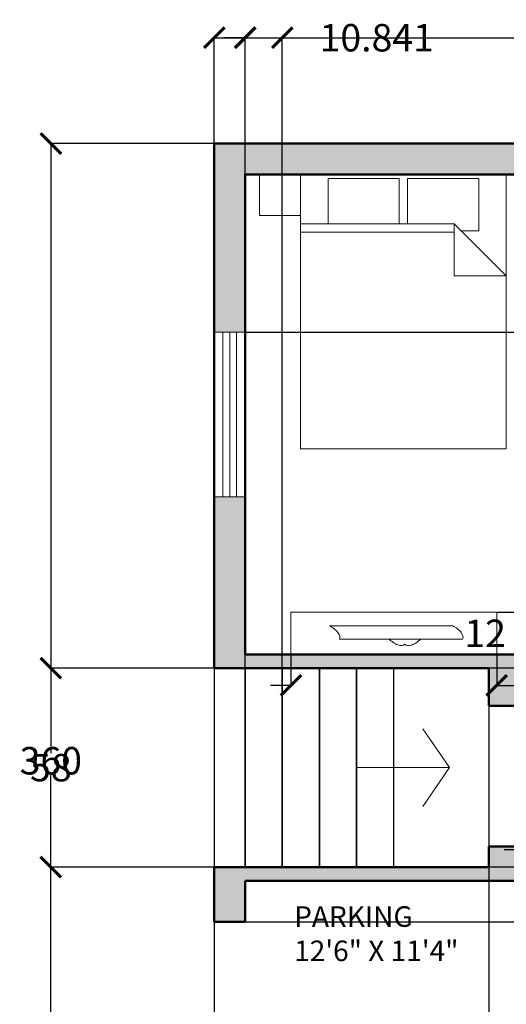
# Model space of a CAD drawing. Units: inches. Extents: x -30 to 744, y -375 to 57.
# Tile 2 of 8: x -26 to 116, y -230 to 57. Entities that reach past the tile are written whole.
import ezdxf

# ---------------------------------------------------------------- set-up
doc = ezdxf.new("R2010")
doc.units = ezdxf.units.IN
doc.header["$MEASUREMENT"] = 0
for name, color, linetype, lineweight in [('A-ANNO-DIMS', 2, 'Continuous', 18), ('A-ANNO-SYMB', 7, 'Continuous', 18), ('A-AREA-IDEN', 7, 'Continuous', 25), ('A-DOOR', 3, 'Continuous', 25), ('A-FLOR-STRS', 7, 'Continuous', 25), ('A-FURN', 8, 'Continuous', 18), ('A-GLAZ', 4, 'Continuous', 18), ('A-WALL', 7, 'Continuous', 50)]:
    doc.layers.add(name, color=color, linetype=linetype, lineweight=lineweight)
doc.layers.add('A-WALL-PATT', color=251, linetype='Continuous', lineweight=13, true_color=0x636466)
doc.styles.get("Standard").update_dxf_attribs({"font": 'arial.ttf'})
doc.dimstyles.get("Standard").update_dxf_attribs({"dimtxt": 8, "dimasz": 6, "dimexe": 0.18, "dimexo": 0.0625, "dimgap": 0.09, "dimtad": 0, "dimtih": 1, "dimtoh": 1, "dimdec": 0, "dimzin": 0, "dimdsep": 46, "dimlunit": 4, "dimtxsty": 'Standard', "dimblk": 'ARCHTICK', "dimcen": 0.09, "dimadec": 0, "dimazin": 0, "dimtfac": 1, "dimtdec": 0, "dimtofl": 0, "dimtmove": 0, "dimatfit": 1, "dimldrblk": 'ARCHTICK', "dimfxl": 1, "dimtolj": 1, "dimtzin": 0, "dimarcsym": 0})

# ---------------------------------------------------------------- blocks, each defined once
blk = doc.blocks.new('*U2')
for p, q in [((0, 0), (0, -6)), ((40, 0), (40, -6))]:
    blk.add_line(p, q)
blk.add_lwpolyline([(0, 0), (34.64, 20), (35.52, 18.48), (0.87, -1.52)], close=True)
blk.add_arc((0, 0), 40, 0, 30)
blk = doc.blocks.new('Bed - Queen')
for p, q in [((0, -80.00003), (0, 0)), ((0, 0), (59.99999, 0)), ((59.99999, 0), (59.99999, -80.00003)), ((7.99999, -1.2), (28.79998, -1.2)), ((7.99999, -14.4), (7.99999, -1.2)), ((28.79998, -1.2), (28.79998, -14.4)), ((31.19999, -1.2), (51.99999, -1.2)), ((31.19999, -14.4), (31.19999, -1.2)), ((51.99999, -1.2), (51.99999, -16.4)), ((0, -14.4), (44.8, -14.4)), ((44.8, -16.8), (0, -16.8)), ((59.99999, -29.6), (44.8, -14.4)), ((44.8, -14.4), (44.8, -29.6)), ((51.99999, -16.4), (46.79936, -16.4)), ((44.8, -29.6), (59.99999, -29.6)), ((59.99999, -80.00003), (0, -80.00003))]:
    blk.add_line(p, q)
blk = doc.blocks.new('WIN-48IN')
for p, q in [((0, 0), (0, 48)), ((0, 48), (9, 48)), ((2.5, 48), (2.5, 0)), ((4.5, 48), (4.5, 0)), ((6.5, 48), (6.5, 0)), ((9, 48), (9, 0)), ((9, 48), (9, 0)), ((9, 0), (0, 0))]:
    blk.add_line(p, q)
blk = doc.blocks.new('TV-CONSOLE-60IN')
blk.add_lwpolyline([(0, 12.35), (60, 12.35), (60, 0), (0, 0)], close=True)
for points in [[(11.23, 8.37), (47.17, 8.37)], [(50.06, 4.48), (14.12, 4.48)]]:
    blk.add_lwpolyline(points)
for centre, major_axis in [((10.57, 6.42), (3.55, -1.95)), ((46.51, 6.42), (3.55, -1.95)), ((36.16, 5.7), (-3.02, -2.7))]:
    blk.add_ellipse(centre, major_axis=major_axis, ratio=0.501579, start_param=0, end_param=1.660459)
at = {"extrusion": (0, 0, -1)}
blk.add_ellipse((30.21, 5.79), major_axis=(2.93, -2.79), ratio=0.501579, start_param=0, end_param=1.660459, dxfattribs=at)
blk = doc.blocks.new('NIGHTSTAND-12IN')
blk.add_lwpolyline([(0, 12), (0, 0), (12, 0), (12, 12)], close=True)
blk = doc.blocks.new('_ArchTick')
at = {"color": 0, "linetype": 'ByBlock', "const_width": 0.15}
blk.add_lwpolyline([(-0.5, -0.5), (0.5, 0.5)], dxfattribs=at)
blk = doc.blocks.new('*D44')
at = {"layer": 'A-ANNO-DIMS', "color": 0, "lineweight": -2, "transparency": 16777216}
for p, q in [((53.6, -128.37), (53.6, -137.48)), ((113.6, -128.37), (113.6, -137.48)), ((53.6, -137.3), (47.6, -137.3)), ((113.6, -137.3), (125.6, -137.3))]:
    blk.add_line(p, q, dxfattribs=at)
at = {"layer": 'Defpoints', "color": 0, "transparency": 16777216}
for p in [(53.6, -128.3), (113.6, -128.3), (113.6, -137.3)]:
    blk.add_point(p, dxfattribs=at)
at = {"layer": 'A-ANNO-DIMS', "color": 0, "lineweight": -2, "transparency": 16777216, "xscale": 6, "yscale": 6, "zscale": 6}
blk.add_blockref('_ArchTick', (53.6, -137.3), dxfattribs=at)
at = {"layer": 'A-ANNO-DIMS', "color": 0, "lineweight": -2, "transparency": 16777216, "xscale": 6, "yscale": 6, "zscale": 6, "rotation": 180}
blk.add_blockref('_ArchTick', (113.6, -137.3), dxfattribs=at)
at = {"layer": 'A-ANNO-DIMS', "color": 0, "transparency": 16777216, "insert": (182.83, -137.3), "char_height": 8, "attachment_point": 5}
blk.add_mtext('\\A1;TV CONSOLE 60 TYP.', dxfattribs=at)
blk = doc.blocks.new('*D45')
at = {"layer": 'A-ANNO-DIMS', "color": 0, "lineweight": -2, "transparency": 16777216}
for p, q in [((113.66, -115.96), (122.78, -115.96)), ((122.6, -115.96), (122.6, -118.02)), ((122.6, -128.3), (122.6, -126.24)), ((113.66, -128.3), (122.78, -128.3))]:
    blk.add_line(p, q, dxfattribs=at)
at = {"layer": 'Defpoints', "color": 0, "transparency": 16777216}
for p in [(113.6, -115.96), (122.6, -115.96), (113.6, -128.3)]:
    blk.add_point(p, dxfattribs=at)
at = {"layer": 'A-ANNO-DIMS', "color": 0, "lineweight": -2, "transparency": 16777216, "xscale": 6, "yscale": 6, "zscale": 6}
for p, rotation in [((122.6, -115.96), 90), ((122.6, -128.3), 270)]:
    blk.add_blockref('_ArchTick', p, dxfattribs=dict(at, rotation=rotation))
at = {"layer": 'A-ANNO-DIMS', "color": 0, "transparency": 16777216, "insert": (122.6, -122.13), "char_height": 8, "attachment_point": 5}
blk.add_mtext('\\A1;12 TYP.', dxfattribs=at)
blk = doc.blocks.new('*D61')
at = {"layer": 'A-ANNO-DIMS', "color": 0, "lineweight": -2, "transparency": 16777216}
for p, q in [((31.17, 20.7), (-16.61, 20.7)), ((-16.43, 20.7), (-16.43, -155.12)), ((-16.43, -339.3), (-16.43, -163.47)), ((31.17, -339.3), (-16.61, -339.3))]:
    blk.add_line(p, q, dxfattribs=at)
at = {"layer": 'Defpoints', "color": 0, "transparency": 16777216}
for p in [(-16.43, 20.7), (31.24, 20.7), (31.24, -339.3)]:
    blk.add_point(p, dxfattribs=at)
at = {"layer": 'A-ANNO-DIMS', "color": 0, "lineweight": -2, "transparency": 16777216, "xscale": 6, "yscale": 6, "zscale": 6}
for p, rotation in [((-16.43, 20.7), 90), ((-16.43, -339.3), 270)]:
    blk.add_blockref('_ArchTick', p, dxfattribs=dict(at, rotation=rotation))
at = {"layer": 'A-ANNO-DIMS', "color": 0, "transparency": 16777216, "insert": (-16.43, -159.3), "char_height": 8, "attachment_point": 5}
blk.add_mtext('\\A1;360', dxfattribs=at)
blk = doc.blocks.new('*D63')
at = {"layer": 'A-ANNO-DIMS', "color": 0, "lineweight": -2, "transparency": 16777216}
for p, q in [((542.17, -132.3), (-16.61, -132.3)), ((-16.43, -132.3), (-16.43, -157.12)), ((-16.43, -190.3), (-16.43, -165.47)), ((542.17, -190.3), (-16.61, -190.3))]:
    blk.add_line(p, q, dxfattribs=at)
at = {"layer": 'Defpoints', "color": 0, "transparency": 16777216}
for p in [(-16.43, -132.3), (542.24, -132.3), (542.24, -190.3)]:
    blk.add_point(p, dxfattribs=at)
at = {"layer": 'A-ANNO-DIMS', "color": 0, "lineweight": -2, "transparency": 16777216, "xscale": 6, "yscale": 6, "zscale": 6}
for p, rotation in [((-16.43, -132.3), 90), ((-16.43, -190.3), 270)]:
    blk.add_blockref('_ArchTick', p, dxfattribs=dict(at, rotation=rotation))
at = {"layer": 'A-ANNO-DIMS', "color": 0, "transparency": 16777216, "insert": (-16.43, -161.3), "char_height": 8, "attachment_point": 5}
blk.add_mtext('\\A1;58', dxfattribs=at)
blk = doc.blocks.new('*D64')
at = {"layer": 'A-ANNO-DIMS', "color": 0, "lineweight": -2, "transparency": 16777216}
for p, q in [((40.3, -206.3), (662.32, -206.3)), ((662.14, -206.3), (662.14, -258.19)), ((662.14, -318.3), (662.14, -266.4)), ((40.3, -318.3), (662.32, -318.3))]:
    blk.add_line(p, q, dxfattribs=at)
at = {"layer": 'Defpoints', "color": 0, "transparency": 16777216}
for p in [(40.24, -206.3), (662.14, -206.3), (40.24, -318.3)]:
    blk.add_point(p, dxfattribs=at)
at = {"layer": 'A-ANNO-DIMS', "color": 0, "lineweight": -2, "transparency": 16777216, "xscale": 6, "yscale": 6, "zscale": 6}
for p, rotation in [((662.14, -206.3), 90), ((662.14, -318.3), 270)]:
    blk.add_blockref('_ArchTick', p, dxfattribs=dict(at, rotation=rotation))
at = {"layer": 'A-ANNO-DIMS', "color": 0, "transparency": 16777216, "insert": (662.14, -262.3), "char_height": 8, "attachment_point": 5}
blk.add_mtext('\\A1;112', dxfattribs=at)
blk = doc.blocks.new('*D65')
at = {"layer": 'A-ANNO-DIMS', "color": 0, "lineweight": -2, "transparency": 16777216}
for p, q in [((31.24, -132.36), (31.24, -370.38)), ((111.31, -143.36), (111.31, -370.38)), ((31.24, -370.2), (57.67, -370.2)), ((111.31, -370.2), (84.88, -370.2))]:
    blk.add_line(p, q, dxfattribs=at)
at = {"layer": 'Defpoints', "color": 0, "transparency": 16777216}
for p in [(31.24, -132.3), (111.31, -143.3), (111.31, -370.2)]:
    blk.add_point(p, dxfattribs=at)
at = {"layer": 'A-ANNO-DIMS', "color": 0, "lineweight": -2, "transparency": 16777216, "xscale": 6, "yscale": 6, "zscale": 6, "rotation": 180}
blk.add_blockref('_ArchTick', (31.24, -370.2), dxfattribs=at)
at = {"layer": 'A-ANNO-DIMS', "color": 0, "lineweight": -2, "transparency": 16777216, "xscale": 6, "yscale": 6, "zscale": 6}
blk.add_blockref('_ArchTick', (111.31, -370.2), dxfattribs=at)
at = {"layer": 'A-ANNO-DIMS', "color": 0, "transparency": 16777216, "insert": (71.27, -370.2), "char_height": 8, "attachment_point": 5}
blk.add_mtext('\\A1;80.08', dxfattribs=at)
blk = doc.blocks.new('*D69')
at = {"layer": 'A-ANNO-DIMS', "color": 0, "lineweight": -2, "transparency": 16777216}
for p, q in [((31.24, 20.77), (31.24, 51.78)), ((233.43, 20.77), (233.43, 51.78)), ((31.24, 51.6), (118.72, 51.6)), ((233.43, 51.6), (145.95, 51.6))]:
    blk.add_line(p, q, dxfattribs=at)
at = {"layer": 'Defpoints', "color": 0, "transparency": 16777216}
for p in [(233.43, 51.6), (31.24, 20.7), (233.43, 20.7)]:
    blk.add_point(p, dxfattribs=at)
at = {"layer": 'A-ANNO-DIMS', "color": 0, "lineweight": -2, "transparency": 16777216, "xscale": 6, "yscale": 6, "zscale": 6, "rotation": 180}
blk.add_blockref('_ArchTick', (31.24, 51.6), dxfattribs=at)
at = {"layer": 'A-ANNO-DIMS', "color": 0, "lineweight": -2, "transparency": 16777216, "xscale": 6, "yscale": 6, "zscale": 6}
blk.add_blockref('_ArchTick', (233.43, 51.6), dxfattribs=at)
at = {"layer": 'A-ANNO-DIMS', "color": 0, "transparency": 16777216, "insert": (132.33, 51.6), "char_height": 8, "attachment_point": 5}
blk.add_mtext('\\A1;202.2', dxfattribs=at)
blk = doc.blocks.new('*D75')
at = {"layer": 'A-ANNO-DIMS', "color": 0, "lineweight": -2, "transparency": 16777216}
for p, q in [((40.3, 11.7), (662.32, 11.7)), ((662.14, 11.7), (662.14, -7.12)), ((662.14, -34.3), (662.14, -15.47)), ((40.3, -34.3), (662.32, -34.3))]:
    blk.add_line(p, q, dxfattribs=at)
at = {"layer": 'Defpoints', "color": 0, "transparency": 16777216}
for p in [(40.24, 11.7), (662.14, 11.7), (40.24, -34.3)]:
    blk.add_point(p, dxfattribs=at)
at = {"layer": 'A-ANNO-DIMS', "color": 0, "lineweight": -2, "transparency": 16777216, "xscale": 6, "yscale": 6, "zscale": 6}
for p, rotation in [((662.14, 11.7), 90), ((662.14, -34.3), 270)]:
    blk.add_blockref('_ArchTick', p, dxfattribs=dict(at, rotation=rotation))
at = {"layer": 'A-ANNO-DIMS', "color": 0, "transparency": 16777216, "insert": (662.14, -11.3), "char_height": 8, "attachment_point": 5}
blk.add_mtext('\\A1;46', dxfattribs=at)
blk = doc.blocks.new('*D81')
at = {"layer": 'A-ANNO-DIMS', "color": 0, "lineweight": -2, "transparency": 16777216}
for p, q in [((40.24, -190.23), (40.24, 51.78)), ((51.08, -190.23), (51.08, 51.78)), ((40.24, 51.6), (34.24, 51.6)), ((51.08, 51.6), (63.08, 51.6))]:
    blk.add_line(p, q, dxfattribs=at)
at = {"layer": 'Defpoints', "color": 0, "transparency": 16777216}
for p in [(51.08, 51.6), (40.24, -190.3), (51.08, -190.3)]:
    blk.add_point(p, dxfattribs=at)
at = {"layer": 'A-ANNO-DIMS', "color": 0, "lineweight": -2, "transparency": 16777216, "xscale": 6, "yscale": 6, "zscale": 6}
blk.add_blockref('_ArchTick', (40.24, 51.6), dxfattribs=at)
at = {"layer": 'A-ANNO-DIMS', "color": 0, "lineweight": -2, "transparency": 16777216, "xscale": 6, "yscale": 6, "zscale": 6, "rotation": 180}
blk.add_blockref('_ArchTick', (51.08, 51.6), dxfattribs=at)
at = {"layer": 'A-ANNO-DIMS', "color": 0, "transparency": 16777216, "insert": (78.62, 51.6), "char_height": 8, "attachment_point": 5}
blk.add_mtext('\\A1;10.841', dxfattribs=at)

msp = doc.modelspace()

# ---------------------------------------------------------------- hatches: boundary and pattern name
at = {"layer": 'A-WALL-PATT'}
h = msp.add_hatch(color=256, dxfattribs=at)
h.dxf.hatch_style = 1
h.paths.add_polyline_path([(40.2356, 11.7031), (204.2356, 11.7031), (204.2356, -24.2969), (208.2356, -24.2969), (208.2356, 11.7031), (233.4275, 11.7031), (233.4275, 20.7031), (31.2356, 20.7031), (31.2356, -34.2969), (40.2356, -34.2969)])
h.paths.add_polyline_path([(40.2356, -82.2969), (31.2356, -82.2969), (31.2356, -132.2969), (40.2356, -132.2969), (51.0767, -132.2969), (111.3137, -132.2969), (111.3137, -143.2969), (120.3137, -143.2969), (120.3137, -132.2969), (156.2356, -132.2969), (156.2356, -128.2969), (113.6001, -128.2969), (113.6001, -128.3034), (53.6001, -128.3034), (40.2356, -128.2969)])
h.paths.add_polyline_path([(302.4681, 20.7031), (257.4275, 20.7031), (257.4275, 11.7031), (286.2356, 11.7031), (286.2356, -60.2969), (208.2356, -60.2969), (208.2356, -54.2969), (204.2356, -54.2969), (204.2356, -64.2969), (208.2356, -64.2969), (286.2356, -64.2969), (286.2356, -128.2969), (264.8954, -128.2969), (208.2356, -128.2969), (204.2356, -128.2969), (198.2356, -128.2969), (198.2356, -132.2969), (290.2356, -132.2969), (290.2356, -128.2969), (290.2356, 11.7031), (302.4681, 11.7031)])
h.paths.add_polyline_path([(405.515, 20.7031), (350.4681, 20.7031), (350.4681, 11.7031), (362.2356, 11.7031), (362.2356, -34.2969), (366.2356, -34.2969), (366.2356, 11.7031), (405.515, 11.7031)])
h.paths.add_polyline_path([(530.2713, 20.7031), (453.515, 20.7031), (453.515, 11.7031), (486.2356, 11.7031), (486.2356, -128.2969), (448.2356, -128.2969), (448.2356, -132.2969), (486.2356, -132.2969), (490.2356, -132.2969), (496.2356, -132.2969), (496.2356, -128.2969), (490.2356, -128.2969), (490.2356, 11.7031), (530.2713, 11.7031)])
h.paths.add_polyline_path([(631.2356, 20.7031), (578.2713, 20.7031), (578.2713, 11.7031), (622.2356, 11.7031), (622.2356, -37.4001), (631.2356, -37.4001)])
h.paths.add_polyline_path([(631.2356, -85.4001), (622.2356, -85.4001), (622.2356, -91.4001), (622.2356, -103.4001), (622.2356, -128.2969), (538.2356, -128.2969), (538.2356, -132.2969), (538.2356, -154.2969), (542.2356, -154.2969), (542.2356, -132.2969), (575.1375, -132.2969), (585.6313, -131.9348), (585.6438, -132.2969), (622.2356, -132.2969), (622.2356, -147.2969), (631.2356, -147.2969)])
h.paths.add_polyline_path([(631.2356, -171.2969), (622.2356, -171.2969), (622.2356, -185.4028), (622.2356, -186.2969), (622.2356, -190.2969), (542.2356, -190.2969), (542.2356, -184.2969), (538.2356, -184.2969), (538.2356, -190.2969), (538.2356, -194.2969), (622.2356, -194.2969), (622.2356, -237.4632), (631.2356, -237.4632)])
h.paths.add_polyline_path([(631.2356, -285.4632), (622.2356, -285.4632), (622.2356, -330.2969), (490.2356, -330.2969), (490.2356, -194.2969), (494.2356, -194.2969), (495.2356, -194.2969), (495.2356, -190.2969), (494.2356, -190.2969), (490.2356, -190.2969), (486.2356, -190.2969), (366.2356, -190.2969), (366.2356, -194.2969), (486.2356, -194.2969), (486.2356, -330.2969), (426.2356, -330.2969), (426.2356, -339.2969), (631.2356, -339.2969)])
h.paths.add_polyline_path([(378.2356, -330.2969), (318.2356, -330.2969), (318.2356, -194.2969), (324.2356, -194.2969), (324.2356, -190.2969), (318.2356, -190.2969), (314.2356, -190.2969), (314.2356, -194.2969), (314.2356, -330.2969), (278.2356, -330.2969), (278.2356, -339.2969), (378.2356, -339.2969)])
h.paths.add_polyline_path([(190.2356, -330.2969), (40.2356, -330.2969), (40.2356, -318.2969), (31.2356, -318.2969), (31.2356, -330.2969), (31.2356, -339.2969), (190.2356, -339.2969)])
h.paths.add_polyline_path([(230.2356, -330.2969), (194.2356, -330.2969), (194.2356, -194.2969), (194.2356, -190.2969), (190.2356, -190.2969), (184.2356, -190.2969), (184.2356, -194.2969), (190.2356, -194.2969), (190.2356, -339.2969), (230.2356, -339.2969)])
h.paths.add_polyline_path([(142.2356, -190.2969), (120.3137, -190.2969), (120.3137, -184.2969), (116.3137, -184.2969), (111.3137, -184.2969), (111.3137, -190.2969), (40.2356, -190.2969), (31.2356, -190.2969), (31.2356, -194.2969), (31.2356, -206.2969), (40.2356, -206.2969), (40.2356, -194.2969), (142.2356, -194.2969)])

# ---------------------------------------------------------------- linework, layer by layer
at = {"layer": 'A-ANNO-SYMB'}
for p, q in [((99.8619, -161.2969), (92.0669, -149.9818)), ((72.759, -161.2969), (99.8619, -161.2969)), ((99.8619, -161.2969), (92.0669, -172.612))]:
    msp.add_line(p, q, dxfattribs=at)
at = {"layer": 'A-FLOR-STRS'}
for points in [[(51.0767, -132.2969), (40.2356, -132.2969), (40.2356, -190.2969), (51.0767, -190.2969)], [(61.9179, -132.2969), (51.0767, -132.2969), (51.0767, -190.2969), (61.9179, -190.2969)], [(72.759, -132.2969), (61.9179, -132.2969), (61.9179, -190.2969), (72.759, -190.2969)], [(83.6001, -132.2969), (72.759, -132.2969), (72.759, -190.2969), (83.6001, -190.2969)]]:
    msp.add_lwpolyline(points, close=True, dxfattribs=at)
at = {"layer": 'A-WALL'}
for p, q in [((40.2356, 11.7031), (204.2356, 11.7031)), ((40.2356, -128.2969), (40.2356, 11.7031)), ((40.2356, -128.2969), (156.2356, -128.2969)), ((40.2356, -132.2969), (31.2356, -132.2969)), ((40.2356, -132.2969), (111.3137, -132.2969)), ((111.3137, -143.2969), (111.3137, -132.2969)), ((120.3137, -143.2969), (111.3137, -143.2969)), ((116.3137, -184.2969), (111.3137, -184.2969)), ((111.3137, -184.2969), (111.3137, -190.2969)), ((120.3137, -184.2969), (116.3137, -184.2969)), ((31.2356, -194.2969), (31.2356, -190.2969)), ((31.2356, -190.2969), (40.2356, -190.2969)), ((111.3137, -190.2969), (40.2356, -190.2969)), ((31.2356, -194.2969), (31.2356, -206.2969)), ((142.2356, -194.2969), (40.2356, -194.2969)), ((40.2356, -206.2969), (40.2356, -194.2969)), ((31.2356, -206.2969), (40.2356, -206.2969))]:
    msp.add_line(p, q, dxfattribs=at)
msp.add_lwpolyline([(31.2356, -132.2969), (31.2356, 20.7031), (631.2356, 20.7031), (631.2356, -339.2969), (190.2356, -339.2969)], dxfattribs=at)

# ---------------------------------------------------------------- block references
at = {"layer": 'A-DOOR', "xscale": 1.05, "yscale": 1.05, "zscale": 1.05, "rotation": 270}
msp.add_blockref('*U2', (122.1137, -143.2969), dxfattribs=at)
at = {"layer": 'A-FURN', "rotation": 90.00000000000021}
msp.add_blockref('NIGHTSTAND-12IN', (56.4058, -0.2964), dxfattribs=at)
at = {"layer": 'A-FURN'}
for name, p in [('Bed - Queen', (56.4059, 11.7031)), ('TV-CONSOLE-60IN', (53.6, -128.303))]:
    msp.add_blockref(name, p, dxfattribs=at)
at = {"layer": 'A-GLAZ'}
msp.add_blockref('WIN-48IN', (31.236, -82.2967), dxfattribs=at)

# ---------------------------------------------------------------- texts
at = {"layer": 'A-AREA-IDEN', "insert": (54.5317, -201.7413), "char_height": 6, "attachment_point": 1}
msp.add_mtext_dynamic_manual_height_columns('PARKING \\P12\'6" X 11\'4"', width=118.375049, gutter_width=1, heights=[0], dxfattribs=at)

# ---------------------------------------------------------------- dimensions: what is measured, and where the dimension line sits
at = {"layer": 'A-ANNO-DIMS'}
for base, p1, p2, override, picture, middle in [((233.4275, 51.6031), (31.2356, 20.7031), (233.4275, 20.7031), {"dimdec": 1, "dimlfac": 1, "dimrnd": 0, "dimzin": 0, "dimdsep": 46, "dimlunit": 2}, '*D69', (132.3315, 51.6031)), ((51.0767, 51.6031), (40.2356, -190.2969), (51.0767, -190.2969), {"dimdec": 3, "dimlfac": 1, "dimrnd": 0, "dimzin": 0, "dimdsep": 46, "dimlunit": 2}, '*D81', (78.6237, 51.6031)), ((111.3137, -370.1969), (31.2356, -132.2969), (111.3137, -143.2969), {"dimdec": 2, "dimlfac": 1, "dimrnd": 0, "dimzin": 0, "dimdsep": 46, "dimlunit": 2}, '*D65', (71.2746, -370.1969))]:
    dim = msp.add_linear_dim(base=base, p1=p1, p2=p2, dimstyle='Standard', override=override, dxfattribs=at)
    dim.commit()
    dim.dimension.update_dxf_attribs({"geometry": picture, "text_midpoint": middle})
for base, p1, p2, picture, middle in [((-16.4253, 20.7031), (31.2356, -339.2969), (31.2356, 20.7031), '*D61', (-16.4253, -159.2969)), ((662.1356, 11.7031), (40.2356, -34.2969), (40.2356, 11.7031), '*D75', (662.1356, -11.2969)), ((-16.4253, -132.2969), (542.2356, -190.2969), (542.2356, -132.2969), '*D63', (-16.4253, -161.2969)), ((662.1356, -206.2969), (40.2356, -318.2969), (40.2356, -206.2969), '*D64', (662.1356, -262.2969))]:
    dim = msp.add_linear_dim(base=base, p1=p1, p2=p2, angle=90, dimstyle='Standard', override={"dimdec": 0, "dimlfac": 1, "dimrnd": 0, "dimzin": 0, "dimdsep": 46, "dimlunit": 2}, dxfattribs=at)
    dim.commit()
    dim.dimension.update_dxf_attribs({"geometry": picture, "text_midpoint": middle})
dim = msp.add_linear_dim(base=(122.6001, -115.9579), p1=(113.6001, -128.3034), p2=(113.6001, -115.9579), angle=90, text='<> TYP.', dimstyle='Standard', override={"dimdec": 0, "dimlfac": 1, "dimrnd": 0, "dimzin": 0, "dimdsep": 46, "dimlunit": 2}, dxfattribs=at)
dim.commit()
dim.dimension.update_dxf_attribs({"geometry": '*D45', "text_midpoint": (122.6001, -122.1306)})
dim = msp.add_linear_dim(base=(113.6001, -137.3034), p1=(53.6001, -128.3034), p2=(113.6001, -128.3034), text='TV CONSOLE <> TYP.', dimstyle='Standard', override={"dimdec": 0, "dimlfac": 1, "dimrnd": 0, "dimzin": 0, "dimdsep": 46, "dimlunit": 2}, dxfattribs=at)
dim.commit()
dim.dimension.update_dxf_attribs({"geometry": '*D44', "text_midpoint": (182.8334, -137.3034)})

doc.saveas('drawing.dxf')
